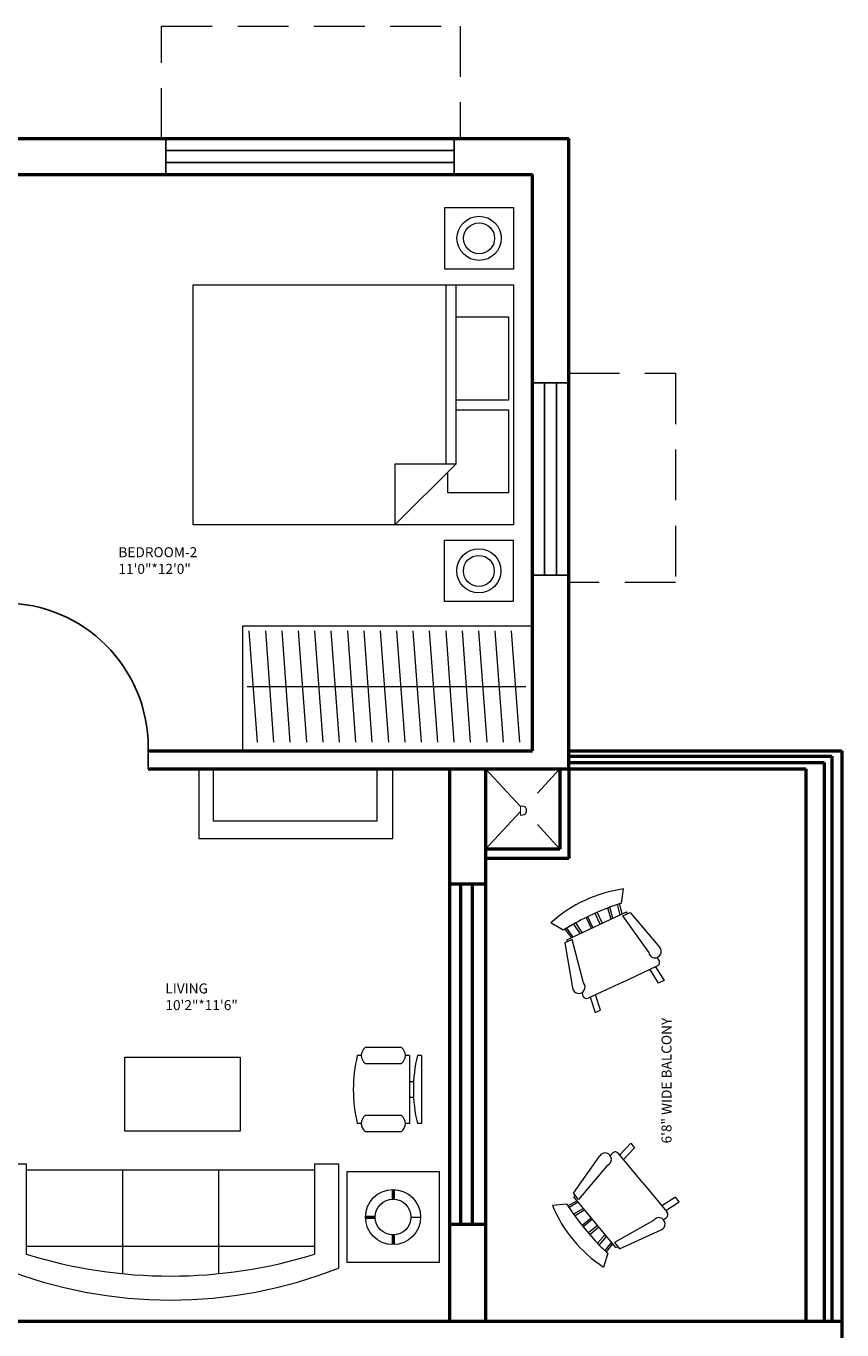
# Model space of a CAD drawing. Units: inches. Extents: x 4795 to 6024, y 2716 to 5025.
# Tile 19 of 19: x 5820 to 6024, y 4676 to 5002. Entities that reach past the tile are written whole.
import ezdxf

# ---------------------------------------------------------------- set-up
doc = ezdxf.new("R2010")
doc.units = ezdxf.units.IN
doc.linetypes.add('DASHED', pattern=[19.05, 12.7, -6.35])
for name, color, linetype, lineweight in [('A-ANNO-TEXT', 7, 'Continuous', 18), ('A-AREA-IDEN', 3, 'Continuous', 18), ('A-DOOR', 4, 'Continuous', 25), ('A-FURN', 8, 'Continuous', 18), ('A-GLAZ', 4, 'Continuous', 25), ('A-WALL', 7, 'Continuous', 50), ('A-WALL-OVHD', 8, 'DASHED', 18)]:
    doc.layers.add(name, color=color, linetype=linetype, lineweight=lineweight)
doc.styles.get("Standard").update_dxf_attribs({"font": 'arial.ttf'})

# ---------------------------------------------------------------- blocks, each defined once
blk = doc.blocks.new('*U2')
for p, q in [((0, 0), (0, -6)), ((40, 0), (40, -6))]:
    blk.add_line(p, q)
blk.add_lwpolyline([(0, 0), (0, 40), (1.75, 40), (1.75, 0)], close=True)
blk.add_arc((0, 0), 40, 0, 90)
blk = doc.blocks.new('Bed - Queen')
for p, q in [((0, -80.00003), (0, 0)), ((0, 0), (59.99999, 0)), ((59.99999, 0), (59.99999, -80.00003)), ((7.99999, -1.2), (28.79998, -1.2)), ((7.99999, -14.4), (7.99999, -1.2)), ((28.79998, -1.2), (28.79998, -14.4)), ((31.19999, -1.2), (51.99999, -1.2)), ((31.19999, -14.4), (31.19999, -1.2)), ((51.99999, -1.2), (51.99999, -16.4)), ((0, -14.4), (44.8, -14.4)), ((59.99999, -29.6), (44.8, -14.4)), ((44.8, -14.4), (44.8, -29.6)), ((44.8, -16.8), (0, -16.8)), ((51.99999, -16.4), (46.79936, -16.4)), ((44.8, -29.6), (59.99999, -29.6)), ((59.99999, -80.00003), (0, -80.00003))]:
    blk.add_line(p, q)
blk = doc.blocks.new('Chair - Rocking')
for p, q in [((-8, -4.5), (-10, -1.5)), ((8, -4.5), (10, -1.5)), ((-7.5, -4.5), (-7, -7)), ((-6.5, -7), (-7.02225, -4.43)), ((-4.5, -7), (-4.96674, -4.19951)), ((-4, -7), (-4.40532, -4.16272)), ((-1.5, -4.05012), (-1.5, -7)), ((-1, -7), (-1, -4.05012)), ((1, -7), (1, -4.04655)), ((1.5, -4.05012), (1.5, -7)), ((4, -7), (4.40187, -4.18694)), ((4.5, -7), (4.96761, -4.19437)), ((6.5, -7), (7, -4.4057)), ((7.5, -4.5), (7, -7)), ((-9, -7.5), (-12, -18.49999)), ((-7, -7.5), (-9, -7.5)), ((-9, -18.49999), (-7, -7.5)), ((-8.23428, -6.99939), (-8.3093, -7.47958)), ((-8.23041, -7), (8.23915, -7)), ((7, -7.5), (9, -7.5)), ((9, -18.49999), (7, -7.5)), ((8.31071, -7.48854), (8.23449, -7.00073)), ((9, -7.5), (12, -18.49999)), ((-10.36644, -20.64523), (-10.5, -21.49999)), ((-9, -22.49999), (-9.5, -26.49999)), ((0, -22.49999), (-9.5, -22.49999)), ((-8, -26.49999), (-7.5, -22.49999)), ((0, -22.49999), (9.5, -22.49999)), ((8, -26.49999), (7.5, -22.49999)), ((9, -22.49999), (9.5, -26.49999)), ((10.5, -21.49999), (10.3575, -20.58798)), ((-9.5, -26.49999), (-8, -26.49999)), ((9.5, -26.49999), (8, -26.49999))]:
    blk.add_line(p, q)
for centre, radius, start, end in [((0, -34.08333), 34.08333, 72.93847, 107.0615), ((0, -68.25004), 64.25, 93.92211, 97.15267), ((0, -68.25004), 64.25, 82.84733, 93.92211), ((-10.5, -18.99999), 1.58114, 161.5651, 18.43495), ((10.5, -18.99999), 1.58114, 161.5651, 18.43495), ((-9.5, -21.49999), 1, 180, 270), ((9.5, -21.49999), 1, 270, 0)]:
    blk.add_arc(centre, radius, start, end)
blk = doc.blocks.new('Sofa - Roundback 7 ft.')
for p, q in [((-12.00002, -32.4421), (-12.00003, -6.5971)), ((11.99997, -32.4421), (11.99998, -6.5971)), ((-36.000027, -34), (-36.000027, -11.4696)), ((35.99998, -34), (35.99998, -11.4696)), ((-35.999844, -13.3819), (35.9998, -13.3819)), ((-36.000027, -32.4421), (35.99998, -32.4421))]:
    blk.add_line(p, q)
for points in [[(-36.000027, -34), (-42.000027, -34), (-42.000027, -8)], [(41.99998, -8), (41.99998, -34), (35.99998, -34)]]:
    blk.add_lwpolyline(points)
for centre, radius, start, end in [((0, -114.25), 114.25, 68.43141, 111.5686), ((-0.00001, -127.1968), 121.1968, 72.72033, 107.2797)]:
    blk.add_arc(centre, radius, start, end)
blk = doc.blocks.new('Chair - Desk')
for p, q in [((-8.5, 0), (-8.5, -1)), ((-8.5, 0), (8.5, 0)), ((8.5, 0), (8.5, -1)), ((-8.5, -3), (-8.5, -4)), ((-8.5, -3), (8.5, -3)), ((-2, -3), (-2, -1.9355)), ((2, -1.9576), (2, -3)), ((8.5, -3), (8.5, -4)), ((-10.5, -5), (-10.5, -14)), ((-6.5, -14), (-6.5, -5)), ((6.5, -5), (6.5, -14)), ((10.5, -14), (10.5, -5)), ((-8.5, -15), (-8.5, -16)), ((8.5, -15), (8.5, -16))]:
    blk.add_line(p, q)
for centre, radius, start, end in [((0, 34.625), 36.625, 256.5803, 283.4197), ((-8.5, -6.5), 2.5, 36.8699, 143.1301), ((8.5, -6.5), 2.5, 36.8699, 143.1301), ((-8.5, -12.5), 2.5, 216.8699, 323.1301), ((0, 19.625), 36.625, 256.5803, 283.4197), ((8.5, -12.5), 2.5, 216.8699, 323.1301)]:
    blk.add_arc(centre, radius, start, end)
blk = doc.blocks.new('WIN-48')
for p, q in [((0, 0), (0, 48)), ((0, 48), (9, 48)), ((3, 0), (3, 48)), ((6, 48), (6, 0)), ((9, 48), (9, 0)), ((9, 0), (0, 0))]:
    blk.add_line(p, q)
blk = doc.blocks.new('WIN-72')
for p, q in [((0, 0), (0, 9)), ((0, 9), (72, 9)), ((72, 9), (72, 0)), ((0, 6), (72, 6)), ((72, 3), (0, 3)), ((72, 0), (0, 0))]:
    blk.add_line(p, q)

msp = doc.modelspace()

# ---------------------------------------------------------------- linework, layer by layer
at = {"layer": 'A-FURN'}
for p, q in [((5874.35, 4820.98), (5874.35, 4852.16)), ((5874.35, 4852.16), (5946.72, 4852.16)), ((5875.89, 4850.95), (5877.94, 4823.11)), ((5879.98, 4850.95), (5882.03, 4823.11)), ((5884.08, 4850.95), (5886.12, 4823.11)), ((5888.17, 4850.95), (5890.22, 4823.11)), ((5892.26, 4850.95), (5894.31, 4823.11)), ((5896.36, 4850.95), (5898.4, 4823.11)), ((5900.45, 4850.95), (5902.5, 4823.11)), ((5904.54, 4850.95), (5906.59, 4823.11)), ((5908.64, 4850.95), (5910.69, 4823.11)), ((5912.73, 4850.95), (5914.78, 4823.11)), ((5916.83, 4850.95), (5918.87, 4823.11)), ((5920.92, 4850.95), (5922.97, 4823.11)), ((5925.01, 4850.95), (5927.06, 4823.11)), ((5929.11, 4850.95), (5931.15, 4823.11)), ((5933.2, 4850.95), (5935.25, 4823.11)), ((5937.29, 4850.95), (5939.34, 4823.11)), ((5941.39, 4850.95), (5943.43, 4823.11)), ((5875.42, 4837.03), (5945.02, 4837.03)), ((5863.34, 4816.48), (5863.34, 4799.03)), ((5866.96, 4816.48), (5866.96, 4803.5)), ((5907.93, 4803.5), (5907.93, 4816.48)), ((5911.85, 4799.03), (5911.85, 4816.48)), ((5866.96, 4803.5), (5907.93, 4803.5)), ((5863.34, 4799.03), (5911.85, 4799.03)), ((5916.32, 4704.47), (5918.73, 4704.47))]:
    msp.add_line(p, q, dxfattribs=at)
for points in [[(5924.79, 4956.67), (5941.91, 4956.67), (5941.91, 4941.33), (5924.79, 4941.33)], [(5924.72, 4873.58), (5941.83, 4873.58), (5941.83, 4858.24), (5924.72, 4858.24)], [(5844.86, 4744.4), (5873.66, 4744.4), (5873.66, 4725.95), (5844.86, 4725.95)], [(5900.38, 4715.83), (5923.34, 4715.83), (5923.34, 4693.12), (5900.38, 4693.12)]]:
    msp.add_lwpolyline(points, close=True, dxfattribs=at)
for centre, radius in [((5933.35, 4949), 5.52), ((5933.35, 4949), 3.86), ((5933.28, 4865.91), 5.52), ((5933.28, 4865.91), 3.86), ((5911.86, 4704.47), 6.88), ((5911.86, 4704.47), 4.47)]:
    msp.add_circle(centre, radius, dxfattribs=at)
at = {"layer": 'A-WALL'}
for p, q in [((5814.72, 4973.98), (5955.72, 4973.98)), ((5955.72, 4816.48), (5955.72, 4973.98)), ((5814.72, 4964.98), (5946.72, 4964.98)), ((5946.72, 4820.98), (5946.72, 4964.98)), ((5850.72, 4820.98), (5946.72, 4820.98)), ((5955.72, 4820.98), (6023.95, 4820.98)), ((5955.72, 4819.65), (6021.44, 4819.65)), ((5955.72, 4818.01), (6019.54, 4818.01)), ((6019.54, 4818.01), (6019.54, 4678.48)), ((6021.44, 4819.65), (6021.44, 4678.48)), ((6023.95, 4820.98), (6023.95, 4673.98)), ((5850.72, 4816.48), (5955.72, 4816.48)), ((5925.95, 4816.48), (5925.95, 4678.48)), ((5934.95, 4816.48), (5934.95, 4678.48)), ((5953.55, 4816.48), (5953.55, 4796.42)), ((5955.72, 4816.48), (6014.95, 4816.48)), ((5955.72, 4816.48), (5955.72, 4794.02)), ((6014.95, 4816.48), (6014.95, 4678.48)), ((5953.55, 4796.42), (5934.95, 4796.42)), ((5955.72, 4794.02), (5934.95, 4794.02)), ((5925.95, 4787.69), (5934.95, 4787.69)), ((5928.74, 4787.69), (5928.74, 4702.69)), ((5931.65, 4787.69), (5931.65, 4702.69)), ((5911.86, 4711.35), (5911.86, 4708.94)), ((5904.98, 4704.47), (5907.39, 4704.47)), ((5925.95, 4702.69), (5934.95, 4702.69)), ((5911.86, 4700.01), (5911.86, 4697.6)), ((5803.72, 4678.48), (5955.72, 4678.48)), ((5955.72, 4678.48), (6023.95, 4678.48))]:
    msp.add_line(p, q, dxfattribs=at)
at = {"layer": 'A-WALL-OVHD'}
for p, q in [((5854.02, 4973.8), (5854.02, 5002.03)), ((5854.02, 5002.03), (5928.61, 5002.03)), ((5928.61, 5002.03), (5928.61, 4973.98)), ((5955.72, 4915.29), (5982.41, 4915.29)), ((5982.41, 4915.29), (5982.41, 4863.02)), ((5982.41, 4863.02), (5955.72, 4863.02)), ((5934.95, 4816.48), (5953.55, 4796.42)), ((5934.95, 4796.42), (5953.55, 4816.48))]:
    msp.add_line(p, q, dxfattribs=at)

# ---------------------------------------------------------------- block references
at = {"layer": 'A-DOOR', "xscale": 0.9, "yscale": 0.9, "zscale": 0.9}
msp.add_blockref('*U2', (5814.72, 4821.88), dxfattribs=at)
at = {"layer": 'A-FURN'}
for name, p, rotation in [('Bed - Queen', (5941.92, 4937.39), 270), ('Chair - Rocking', (5959.73, 4783.59), 24.98478846597024), ('Chair - Desk', (5918.94, 4736.34), 270), ('Chair - Rocking', (5956.89, 4698.69), 129.6958839725731), ('Sofa - Roundback 7 ft.', (5856.28, 4683.73), 180)]:
    msp.add_blockref(name, p, dxfattribs=dict(at, rotation=rotation))
at = {"layer": 'A-GLAZ', "rotation": 180}
msp.add_blockref('WIN-72', (5927.14, 4973.98), dxfattribs=at)
at = {"layer": 'A-GLAZ'}
msp.add_blockref('WIN-48', (5946.72, 4864.88), dxfattribs=at)

# ---------------------------------------------------------------- texts
at = {"layer": 'A-ANNO-TEXT', "insert": (5943.19, 4807.28), "char_height": 2.5, "attachment_point": 1}
msp.add_mtext_dynamic_manual_height_columns('D', width=3.1314, gutter_width=12.5, heights=[0], dxfattribs=at)
at = {"layer": 'A-AREA-IDEN', "char_height": 2.5, "attachment_point": 1}
for s, width, insert in [('BEDROOM-2\\P11\'0"*12\'0"', 58.0649, (5843.29, 4871.83)), ('LIVING\\P10\'2"*11\'6"', 61.8132, (5855.02, 4762.84))]:
    msp.add_mtext_dynamic_manual_height_columns(s, width=width, gutter_width=12.5, heights=[0], dxfattribs=dict(at, insert=insert))
at = {"layer": 'A-AREA-IDEN', "insert": (5978.9, 4722.87), "char_height": 2.5, "attachment_point": 1, "rotation": 90}
msp.add_mtext_dynamic_manual_height_columns('6\'8" WIDE BALCONY', width=55.0719, gutter_width=12.5, heights=[0], dxfattribs=at)

doc.saveas('drawing.dxf')
